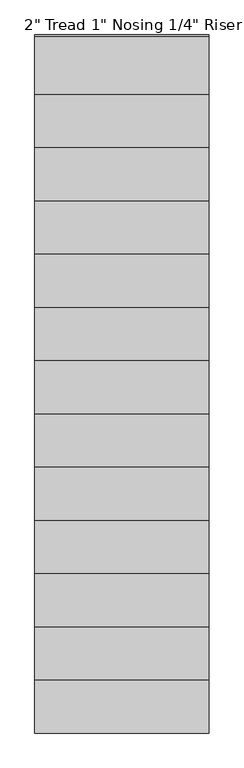
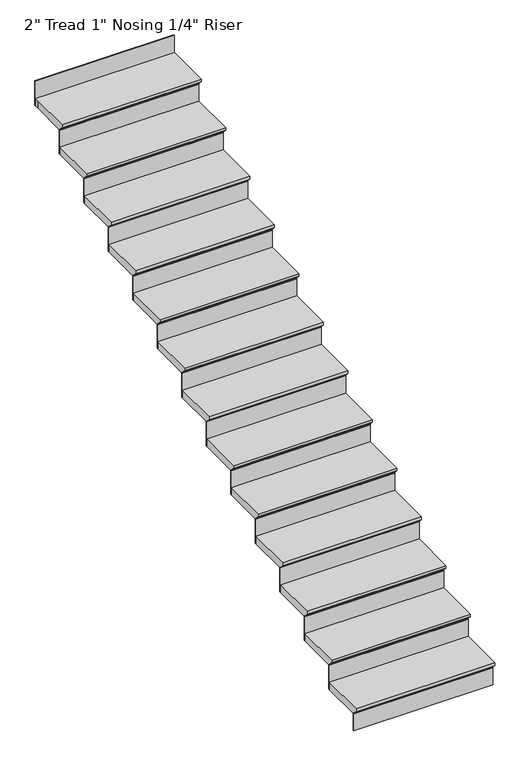
"""IFC4 building model written with IfcOpenShell, lengths in millimetres: stair flight geometry."""

from ifc_helpers import new_model, si_unit, origin, place, context, project, spatial, faceted_brep, source, transform, mapped, element, save


def stair_flight_80be26fe(model_context):
    return source(origin(), model_context, "Body", "Brep", [
        faceted_brep([(-2703.0415084, -23154.3851539, 46720.9005799), (-2703.0415084, -23154.3851539, 46739.9505799), (-3617.4415084, -23154.3851539, 46739.9505799), (-3617.4415084, -23154.3851539, 46720.9005799), (-2703.0415084, -23128.9851539, 46695.5005799), (-3617.4415084, -23128.9851539, 46695.5005799), (-2703.0415084, -22849.5851539, 46739.9505799), (-3617.4415084, -22849.5851539, 46739.9505799), (-3617.4415084, -23128.9851539, 46689.1505799), (-3617.4415084, -22849.5851539, 46689.1505799), (-2703.0415084, -22849.5851539, 46689.1505799), (-2703.0415084, -23128.9851539, 46689.1505799)], [[[0, 1, 2, 3]], [[4, 0, 3, 5]], [[2, 1, 6, 7]], [[8, 9, 10, 11]], [[2, 7, 9, 8, 5, 3]], [[8, 11, 4, 5]], [[6, 1, 0, 4, 11, 10]], [[7, 6, 10, 9]]]),
        faceted_brep([(-2703.0415084, -23128.9851539, 46689.1505799), (-2703.0415084, -23128.9851539, 46570.6172466), (-2703.0415084, -23122.6351539, 46570.6172466), (-2703.0415084, -23122.6351539, 46689.1505799), (-3617.4415084, -23128.9851539, 46689.1505799), (-3617.4415084, -23122.6351539, 46689.1505799), (-3617.4415084, -23122.6351539, 46570.6172466), (-3617.4415084, -23128.9851539, 46570.6172466)], [[[0, 1, 2, 3]], [[4, 5, 6, 7]], [[1, 0, 4, 7]], [[2, 1, 7, 6]], [[3, 2, 6, 5]], [[0, 3, 5, 4]]]),
        faceted_brep([(-2703.0415084, -22849.5851539, 46858.4839133), (-2703.0415084, -22849.5851539, 46689.1505799), (-2703.0415084, -22843.2351539, 46689.1505799), (-2703.0415084, -22843.2351539, 46858.4839133), (-3617.4415084, -22849.5851539, 46858.4839133), (-3617.4415084, -22843.2351539, 46858.4839133), (-3617.4415084, -22843.2351539, 46689.1505799), (-3617.4415084, -22849.5851539, 46689.1505799)], [[[0, 1, 2, 3]], [[4, 5, 6, 7]], [[1, 0, 4, 7]], [[2, 1, 7, 6]], [[3, 2, 6, 5]], [[0, 3, 5, 4]]]),
        faceted_brep([(-3617.4415084, -22874.9851539, 46909.2839133), (-2703.0415084, -22874.9851539, 46909.2839133), (-2703.0415084, -22570.1851539, 46909.2839133), (-3617.4415084, -22570.1851539, 46909.2839133), (-3617.4415084, -22849.5851539, 46858.4839133), (-3617.4415084, -22570.1851539, 46858.4839133), (-2703.0415084, -22570.1851539, 46858.4839133), (-2703.0415084, -22849.5851539, 46858.4839133), (-3617.4415084, -22849.5851539, 46864.8339133), (-3617.4415084, -22874.9851539, 46890.2339133), (-2703.0415084, -22849.5851539, 46864.8339133), (-2703.0415084, -22874.9851539, 46890.2339133)], [[[0, 1, 2, 3]], [[4, 5, 6, 7]], [[0, 3, 5, 4, 8, 9]], [[4, 7, 10, 8]], [[2, 1, 11, 10, 7, 6]], [[3, 2, 6, 5]], [[11, 1, 0, 9]], [[10, 11, 9, 8]]]),
        faceted_brep([(-2703.0415084, -22570.1851539, 47027.8172466), (-2703.0415084, -22570.1851539, 46858.4839133), (-2703.0415084, -22563.8351539, 46858.4839133), (-2703.0415084, -22563.8351539, 47027.8172466), (-3617.4415084, -22570.1851539, 47027.8172466), (-3617.4415084, -22563.8351539, 47027.8172466), (-3617.4415084, -22563.8351539, 46858.4839133), (-3617.4415084, -22570.1851539, 46858.4839133)], [[[0, 1, 2, 3]], [[4, 5, 6, 7]], [[1, 0, 4, 7]], [[2, 1, 7, 6]], [[3, 2, 6, 5]], [[0, 3, 5, 4]]]),
        faceted_brep([(-3617.4415084, -22595.5851539, 47078.6172466), (-2703.0415084, -22595.5851539, 47078.6172466), (-2703.0415084, -22290.7851539, 47078.6172466), (-3617.4415084, -22290.7851539, 47078.6172466), (-3617.4415084, -22570.1851539, 47027.8172466), (-3617.4415084, -22290.7851539, 47027.8172466), (-2703.0415084, -22290.7851539, 47027.8172466), (-2703.0415084, -22570.1851539, 47027.8172466), (-3617.4415084, -22570.1851539, 47034.1672466), (-3617.4415084, -22595.5851539, 47059.5672466), (-2703.0415084, -22570.1851539, 47034.1672466), (-2703.0415084, -22595.5851539, 47059.5672466)], [[[0, 1, 2, 3]], [[4, 5, 6, 7]], [[0, 3, 5, 4, 8, 9]], [[4, 7, 10, 8]], [[2, 1, 11, 10, 7, 6]], [[3, 2, 6, 5]], [[11, 1, 0, 9]], [[10, 11, 9, 8]]]),
        faceted_brep([(-2703.0415084, -22290.7851539, 47197.1505799), (-2703.0415084, -22290.7851539, 47027.8172466), (-2703.0415084, -22284.4351539, 47027.8172466), (-2703.0415084, -22284.4351539, 47197.1505799), (-3617.4415084, -22290.7851539, 47197.1505799), (-3617.4415084, -22284.4351539, 47197.1505799), (-3617.4415084, -22284.4351539, 47027.8172466), (-3617.4415084, -22290.7851539, 47027.8172466)], [[[0, 1, 2, 3]], [[4, 5, 6, 7]], [[1, 0, 4, 7]], [[2, 1, 7, 6]], [[3, 2, 6, 5]], [[0, 3, 5, 4]]]),
        faceted_brep([(-3617.4415084, -22316.1851539, 47247.9505799), (-2703.0415084, -22316.1851539, 47247.9505799), (-2703.0415084, -22011.3851539, 47247.9505799), (-3617.4415084, -22011.3851539, 47247.9505799), (-3617.4415084, -22290.7851539, 47197.1505799), (-3617.4415084, -22011.3851539, 47197.1505799), (-2703.0415084, -22011.3851539, 47197.1505799), (-2703.0415084, -22290.7851539, 47197.1505799), (-3617.4415084, -22290.7851539, 47203.5005799), (-3617.4415084, -22316.1851539, 47228.9005799), (-2703.0415084, -22290.7851539, 47203.5005799), (-2703.0415084, -22316.1851539, 47228.9005799)], [[[0, 1, 2, 3]], [[4, 5, 6, 7]], [[0, 3, 5, 4, 8, 9]], [[4, 7, 10, 8]], [[2, 1, 11, 10, 7, 6]], [[3, 2, 6, 5]], [[11, 1, 0, 9]], [[10, 11, 9, 8]]]),
        faceted_brep([(-2703.0415084, -22011.3851539, 47366.4839133), (-2703.0415084, -22011.3851539, 47197.1505799), (-2703.0415084, -22005.0351539, 47197.1505799), (-2703.0415084, -22005.0351539, 47366.4839133), (-3617.4415084, -22011.3851539, 47366.4839133), (-3617.4415084, -22005.0351539, 47366.4839133), (-3617.4415084, -22005.0351539, 47197.1505799), (-3617.4415084, -22011.3851539, 47197.1505799)], [[[0, 1, 2, 3]], [[4, 5, 6, 7]], [[1, 0, 4, 7]], [[2, 1, 7, 6]], [[3, 2, 6, 5]], [[0, 3, 5, 4]]]),
        faceted_brep([(-3617.4415084, -22036.7851539, 47417.2839133), (-2703.0415084, -22036.7851539, 47417.2839133), (-2703.0415084, -21731.9851539, 47417.2839133), (-3617.4415084, -21731.9851539, 47417.2839133), (-3617.4415084, -22011.3851539, 47366.4839133), (-3617.4415084, -21731.9851539, 47366.4839133), (-2703.0415084, -21731.9851539, 47366.4839133), (-2703.0415084, -22011.3851539, 47366.4839133), (-3617.4415084, -22011.3851539, 47372.8339133), (-3617.4415084, -22036.7851539, 47398.2339133), (-2703.0415084, -22011.3851539, 47372.8339133), (-2703.0415084, -22036.7851539, 47398.2339133)], [[[0, 1, 2, 3]], [[4, 5, 6, 7]], [[0, 3, 5, 4, 8, 9]], [[4, 7, 10, 8]], [[2, 1, 11, 10, 7, 6]], [[3, 2, 6, 5]], [[11, 1, 0, 9]], [[10, 11, 9, 8]]]),
        faceted_brep([(-2703.0415084, -21731.9851539, 47535.8172466), (-2703.0415084, -21731.9851539, 47366.4839133), (-2703.0415084, -21725.6351539, 47366.4839133), (-2703.0415084, -21725.6351539, 47535.8172466), (-3617.4415084, -21731.9851539, 47535.8172466), (-3617.4415084, -21725.6351539, 47535.8172466), (-3617.4415084, -21725.6351539, 47366.4839133), (-3617.4415084, -21731.9851539, 47366.4839133)], [[[0, 1, 2, 3]], [[4, 5, 6, 7]], [[1, 0, 4, 7]], [[2, 1, 7, 6]], [[3, 2, 6, 5]], [[0, 3, 5, 4]]]),
        faceted_brep([(-3617.4415084, -21757.3851539, 47586.6172466), (-2703.0415084, -21757.3851539, 47586.6172466), (-2703.0415084, -21452.5851539, 47586.6172466), (-3617.4415084, -21452.5851539, 47586.6172466), (-3617.4415084, -21731.9851539, 47535.8172466), (-3617.4415084, -21452.5851539, 47535.8172466), (-2703.0415084, -21452.5851539, 47535.8172466), (-2703.0415084, -21731.9851539, 47535.8172466), (-3617.4415084, -21731.9851539, 47542.1672466), (-3617.4415084, -21757.3851539, 47567.5672466), (-2703.0415084, -21731.9851539, 47542.1672466), (-2703.0415084, -21757.3851539, 47567.5672466)], [[[0, 1, 2, 3]], [[4, 5, 6, 7]], [[0, 3, 5, 4, 8, 9]], [[4, 7, 10, 8]], [[2, 1, 11, 10, 7, 6]], [[3, 2, 6, 5]], [[11, 1, 0, 9]], [[10, 11, 9, 8]]]),
        faceted_brep([(-2703.0415084, -21452.5851539, 47705.1505799), (-2703.0415084, -21452.5851539, 47535.8172466), (-2703.0415084, -21446.2351539, 47535.8172466), (-2703.0415084, -21446.2351539, 47705.1505799), (-3617.4415084, -21452.5851539, 47705.1505799), (-3617.4415084, -21446.2351539, 47705.1505799), (-3617.4415084, -21446.2351539, 47535.8172466), (-3617.4415084, -21452.5851539, 47535.8172466)], [[[0, 1, 2, 3]], [[4, 5, 6, 7]], [[1, 0, 4, 7]], [[2, 1, 7, 6]], [[3, 2, 6, 5]], [[0, 3, 5, 4]]]),
        faceted_brep([(-3617.4415084, -21477.9851539, 47755.9505799), (-2703.0415084, -21477.9851539, 47755.9505799), (-2703.0415084, -21173.1851539, 47755.9505799), (-3617.4415084, -21173.1851539, 47755.9505799), (-3617.4415084, -21452.5851539, 47705.1505799), (-3617.4415084, -21173.1851539, 47705.1505799), (-2703.0415084, -21173.1851539, 47705.1505799), (-2703.0415084, -21452.5851539, 47705.1505799), (-3617.4415084, -21452.5851539, 47711.5005799), (-3617.4415084, -21477.9851539, 47736.9005799), (-2703.0415084, -21452.5851539, 47711.5005799), (-2703.0415084, -21477.9851539, 47736.9005799)], [[[0, 1, 2, 3]], [[4, 5, 6, 7]], [[0, 3, 5, 4, 8, 9]], [[4, 7, 10, 8]], [[2, 1, 11, 10, 7, 6]], [[3, 2, 6, 5]], [[11, 1, 0, 9]], [[10, 11, 9, 8]]]),
        faceted_brep([(-2703.0415084, -21173.1851539, 47874.4839133), (-2703.0415084, -21173.1851539, 47705.1505799), (-2703.0415084, -21166.8351539, 47705.1505799), (-2703.0415084, -21166.8351539, 47874.4839133), (-3617.4415084, -21173.1851539, 47874.4839133), (-3617.4415084, -21166.8351539, 47874.4839133), (-3617.4415084, -21166.8351539, 47705.1505799), (-3617.4415084, -21173.1851539, 47705.1505799)], [[[0, 1, 2, 3]], [[4, 5, 6, 7]], [[1, 0, 4, 7]], [[2, 1, 7, 6]], [[3, 2, 6, 5]], [[0, 3, 5, 4]]]),
        faceted_brep([(-3617.4415084, -21198.5851539, 47925.2839133), (-2703.0415084, -21198.5851539, 47925.2839133), (-2703.0415084, -20893.7851539, 47925.2839133), (-3617.4415084, -20893.7851539, 47925.2839133), (-3617.4415084, -21173.1851539, 47874.4839133), (-3617.4415084, -20893.7851539, 47874.4839133), (-2703.0415084, -20893.7851539, 47874.4839133), (-2703.0415084, -21173.1851539, 47874.4839133), (-3617.4415084, -21173.1851539, 47880.8339133), (-3617.4415084, -21198.5851539, 47906.2339133), (-2703.0415084, -21173.1851539, 47880.8339133), (-2703.0415084, -21198.5851539, 47906.2339133)], [[[0, 1, 2, 3]], [[4, 5, 6, 7]], [[0, 3, 5, 4, 8, 9]], [[4, 7, 10, 8]], [[2, 1, 11, 10, 7, 6]], [[3, 2, 6, 5]], [[11, 1, 0, 9]], [[10, 11, 9, 8]]]),
        faceted_brep([(-2703.0415084, -20893.7851539, 48043.8172466), (-2703.0415084, -20893.7851539, 47874.4839133), (-2703.0415084, -20887.4351539, 47874.4839133), (-2703.0415084, -20887.4351539, 48043.8172466), (-3617.4415084, -20893.7851539, 48043.8172466), (-3617.4415084, -20887.4351539, 48043.8172466), (-3617.4415084, -20887.4351539, 47874.4839133), (-3617.4415084, -20893.7851539, 47874.4839133)], [[[0, 1, 2, 3]], [[4, 5, 6, 7]], [[1, 0, 4, 7]], [[2, 1, 7, 6]], [[3, 2, 6, 5]], [[0, 3, 5, 4]]]),
        faceted_brep([(-3617.4415084, -20919.1851539, 48094.6172466), (-2703.0415084, -20919.1851539, 48094.6172466), (-2703.0415084, -20614.3851539, 48094.6172466), (-3617.4415084, -20614.3851539, 48094.6172466), (-3617.4415084, -20893.7851539, 48043.8172466), (-3617.4415084, -20614.3851539, 48043.8172466), (-2703.0415084, -20614.3851539, 48043.8172466), (-2703.0415084, -20893.7851539, 48043.8172466), (-3617.4415084, -20893.7851539, 48050.1672466), (-3617.4415084, -20919.1851539, 48075.5672466), (-2703.0415084, -20893.7851539, 48050.1672466), (-2703.0415084, -20919.1851539, 48075.5672466)], [[[0, 1, 2, 3]], [[4, 5, 6, 7]], [[0, 3, 5, 4, 8, 9]], [[4, 7, 10, 8]], [[2, 1, 11, 10, 7, 6]], [[3, 2, 6, 5]], [[11, 1, 0, 9]], [[10, 11, 9, 8]]]),
        faceted_brep([(-2703.0415084, -20614.3851539, 48213.1505799), (-2703.0415084, -20614.3851539, 48043.8172466), (-2703.0415084, -20608.0351539, 48043.8172466), (-2703.0415084, -20608.0351539, 48213.1505799), (-3617.4415084, -20614.3851539, 48213.1505799), (-3617.4415084, -20608.0351539, 48213.1505799), (-3617.4415084, -20608.0351539, 48043.8172466), (-3617.4415084, -20614.3851539, 48043.8172466)], [[[0, 1, 2, 3]], [[4, 5, 6, 7]], [[1, 0, 4, 7]], [[2, 1, 7, 6]], [[3, 2, 6, 5]], [[0, 3, 5, 4]]]),
        faceted_brep([(-3617.4415084, -20639.7851539, 48263.9505799), (-2703.0415084, -20639.7851539, 48263.9505799), (-2703.0415084, -20334.9851539, 48263.9505799), (-3617.4415084, -20334.9851539, 48263.9505799), (-3617.4415084, -20614.3851539, 48213.1505799), (-3617.4415084, -20334.9851539, 48213.1505799), (-2703.0415084, -20334.9851539, 48213.1505799), (-2703.0415084, -20614.3851539, 48213.1505799), (-3617.4415084, -20614.3851539, 48219.5005799), (-3617.4415084, -20639.7851539, 48244.9005799), (-2703.0415084, -20614.3851539, 48219.5005799), (-2703.0415084, -20639.7851539, 48244.9005799)], [[[0, 1, 2, 3]], [[4, 5, 6, 7]], [[0, 3, 5, 4, 8, 9]], [[4, 7, 10, 8]], [[2, 1, 11, 10, 7, 6]], [[3, 2, 6, 5]], [[11, 1, 0, 9]], [[10, 11, 9, 8]]]),
        faceted_brep([(-2703.0415084, -20334.9851539, 48382.4839133), (-2703.0415084, -20334.9851539, 48213.1505799), (-2703.0415084, -20328.6351539, 48213.1505799), (-2703.0415084, -20328.6351539, 48382.4839133), (-3617.4415084, -20334.9851539, 48382.4839133), (-3617.4415084, -20328.6351539, 48382.4839133), (-3617.4415084, -20328.6351539, 48213.1505799), (-3617.4415084, -20334.9851539, 48213.1505799)], [[[0, 1, 2, 3]], [[4, 5, 6, 7]], [[1, 0, 4, 7]], [[2, 1, 7, 6]], [[3, 2, 6, 5]], [[0, 3, 5, 4]]]),
        faceted_brep([(-3617.4415084, -20360.3851539, 48433.2839133), (-2703.0415084, -20360.3851539, 48433.2839133), (-2703.0415084, -20055.5851539, 48433.2839133), (-3617.4415084, -20055.5851539, 48433.2839133), (-3617.4415084, -20334.9851539, 48382.4839133), (-3617.4415084, -20055.5851539, 48382.4839133), (-2703.0415084, -20055.5851539, 48382.4839133), (-2703.0415084, -20334.9851539, 48382.4839133), (-3617.4415084, -20334.9851539, 48388.8339133), (-3617.4415084, -20360.3851539, 48414.2339133), (-2703.0415084, -20334.9851539, 48388.8339133), (-2703.0415084, -20360.3851539, 48414.2339133)], [[[0, 1, 2, 3]], [[4, 5, 6, 7]], [[0, 3, 5, 4, 8, 9]], [[4, 7, 10, 8]], [[2, 1, 11, 10, 7, 6]], [[3, 2, 6, 5]], [[11, 1, 0, 9]], [[10, 11, 9, 8]]]),
        faceted_brep([(-2703.0415084, -20055.5851539, 48551.8172466), (-2703.0415084, -20055.5851539, 48382.4839133), (-2703.0415084, -20049.2351539, 48382.4839133), (-2703.0415084, -20049.2351539, 48551.8172466), (-3617.4415084, -20055.5851539, 48551.8172466), (-3617.4415084, -20049.2351539, 48551.8172466), (-3617.4415084, -20049.2351539, 48382.4839133), (-3617.4415084, -20055.5851539, 48382.4839133)], [[[0, 1, 2, 3]], [[4, 5, 6, 7]], [[1, 0, 4, 7]], [[2, 1, 7, 6]], [[3, 2, 6, 5]], [[0, 3, 5, 4]]]),
        faceted_brep([(-3617.4415084, -20080.9851539, 48602.6172466), (-2703.0415084, -20080.9851539, 48602.6172466), (-2703.0415084, -19776.1851539, 48602.6172466), (-3617.4415084, -19776.1851539, 48602.6172466), (-3617.4415084, -20055.5851539, 48551.8172466), (-3617.4415084, -19776.1851539, 48551.8172466), (-2703.0415084, -19776.1851539, 48551.8172466), (-2703.0415084, -20055.5851539, 48551.8172466), (-3617.4415084, -20055.5851539, 48558.1672466), (-3617.4415084, -20080.9851539, 48583.5672466), (-2703.0415084, -20055.5851539, 48558.1672466), (-2703.0415084, -20080.9851539, 48583.5672466)], [[[0, 1, 2, 3]], [[4, 5, 6, 7]], [[0, 3, 5, 4, 8, 9]], [[4, 7, 10, 8]], [[2, 1, 11, 10, 7, 6]], [[3, 2, 6, 5]], [[11, 1, 0, 9]], [[10, 11, 9, 8]]]),
        faceted_brep([(-2703.0415084, -19496.7851539, 48890.4839133), (-2703.0415084, -19496.7851539, 48721.1505799), (-2703.0415084, -19490.4351539, 48721.1505799), (-2703.0415084, -19490.4351539, 48890.4839133), (-3617.4415084, -19496.7851539, 48890.4839133), (-3617.4415084, -19490.4351539, 48890.4839133), (-3617.4415084, -19490.4351539, 48721.1505799), (-3617.4415084, -19496.7851539, 48721.1505799)], [[[0, 1, 2, 3]], [[4, 5, 6, 7]], [[1, 0, 4, 7]], [[2, 1, 7, 6]], [[3, 2, 6, 5]], [[0, 3, 5, 4]]]),
        faceted_brep([(-2703.0415084, -19776.1851539, 48721.1505799), (-2703.0415084, -19776.1851539, 48551.8172466), (-2703.0415084, -19769.8351539, 48551.8172466), (-2703.0415084, -19769.8351539, 48721.1505799), (-3617.4415084, -19776.1851539, 48721.1505799), (-3617.4415084, -19769.8351539, 48721.1505799), (-3617.4415084, -19769.8351539, 48551.8172466), (-3617.4415084, -19776.1851539, 48551.8172466)], [[[0, 1, 2, 3]], [[4, 5, 6, 7]], [[1, 0, 4, 7]], [[2, 1, 7, 6]], [[3, 2, 6, 5]], [[0, 3, 5, 4]]]),
        faceted_brep([(-3617.4415084, -19496.7851539, 48771.9505799), (-3617.4415084, -19522.1851539, 48771.9505799), (-3617.4415084, -19801.5851539, 48771.9505799), (-2703.0415084, -19801.5851539, 48771.9505799), (-2703.0415084, -19496.7851539, 48771.9505799), (-3617.4415084, -19522.1851539, 48721.1505799), (-3617.4415084, -19496.7851539, 48721.1505799), (-2703.0415084, -19496.7851539, 48721.1505799), (-2703.0415084, -19776.1851539, 48721.1505799), (-3617.4415084, -19776.1851539, 48721.1505799), (-3617.4415084, -19776.1851539, 48727.5005799), (-3617.4415084, -19801.5851539, 48752.9005799), (-2703.0415084, -19776.1851539, 48727.5005799), (-2703.0415084, -19801.5851539, 48752.9005799)], [[[0, 1, 2, 3, 4]], [[5, 6, 7, 8, 9]], [[1, 0, 6, 5]], [[2, 1, 5, 9, 10, 11]], [[9, 8, 12, 10]], [[4, 3, 13, 12, 8, 7]], [[0, 4, 7, 6]], [[13, 3, 2, 11]], [[12, 13, 11, 10]]]),
    ])


if __name__ == "__main__":
    model = new_model("IFC4")
    model_context = context("Model", 3, world=origin())
    ifc_project = project(units=[si_unit("LENGTHUNIT", "METRE", prefix="MILLI")], contexts=[model_context])
    site = spatial("IfcSite", under=ifc_project)
    building = spatial("IfcBuilding", under=site)
    placement = place(None, origin())
    stair_flight_shape = stair_flight_80be26fe(model_context)
    element("IfcStairFlight", 1, ObjectType="2\" Tread 1\" Nosing 1/4\" Riser", at=placement, inside=building, context=model_context, shape_type="MappedRepresentation", body=[
        mapped(stair_flight_shape, transform((0.0, 0.0, 0.0), x_axis=(1.0, 0.0, 0.0), y_axis=(0.0, 1.0, 0.0), z_axis=(0.0, 0.0, 1.0))),
    ])
    save(model, "model.ifc")
